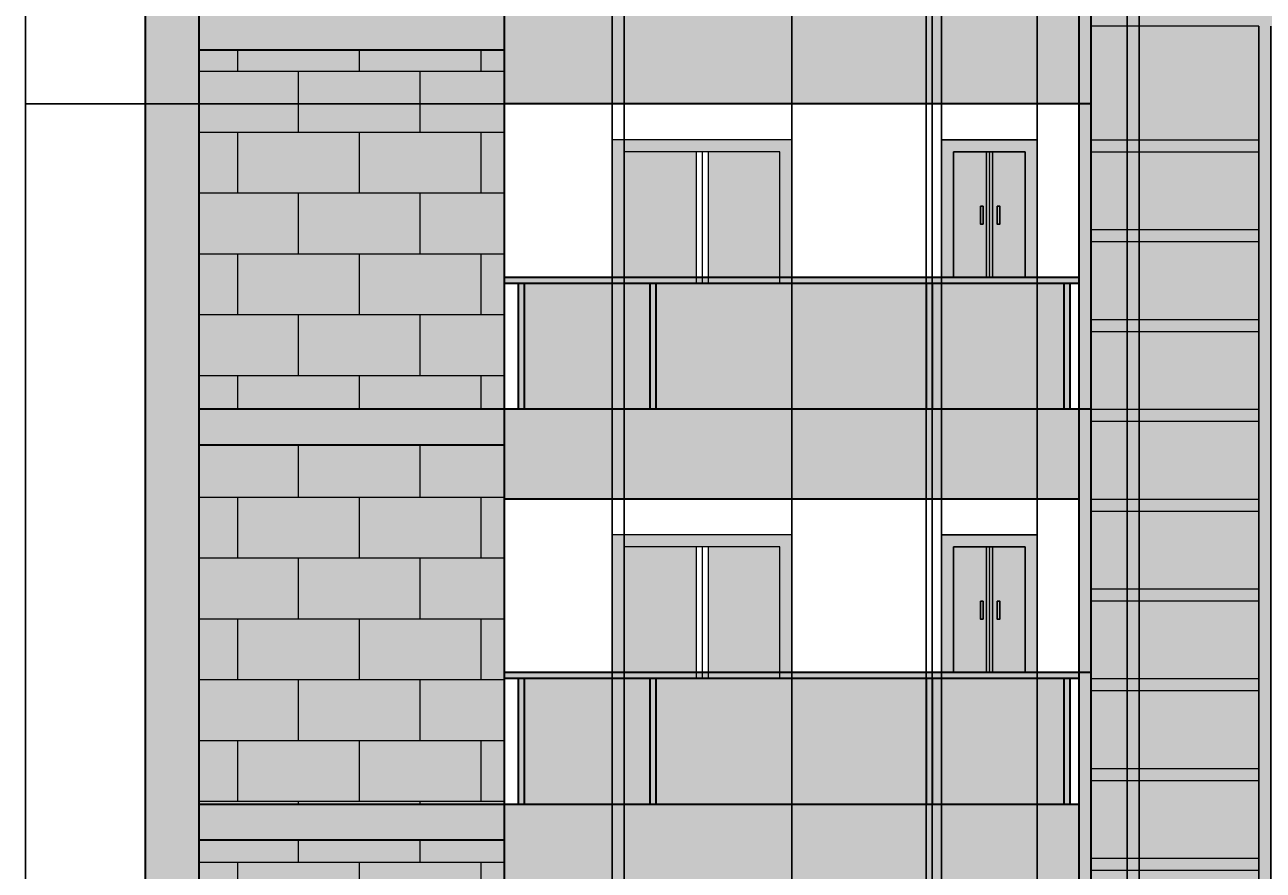
# Model space of a CAD drawing. Units: inches. Extents: x 2794 to 3619, y 522 to 1397.
# Tile 7 of 10: x 2794 to 3208, y 973 to 1255. Entities that reach past the tile are written whole.
import ezdxf

# ---------------------------------------------------------------- set-up
doc = ezdxf.new("R2010")
doc.units = ezdxf.units.IN
for name, color, linetype, lineweight in [('A-ANNO-DIMS', 2, 'Continuous', 18), ('A-DOOR', 3, 'Continuous', 25), ('A-ELEV', 7, 'Continuous', 35), ('A-ELEV-PATT', 8, 'Continuous', 13), ('A-GLAZ', 4, 'Continuous', 18)]:
    doc.layers.add(name, color=color, linetype=linetype, lineweight=lineweight)
doc.styles.get("Standard").update_dxf_attribs({"font": 'arial.ttf'})
doc.dimstyles.get("Standard").update_dxf_attribs({"dimtxt": 0.18, "dimasz": 0.18, "dimexe": 0.18, "dimexo": 0.0625, "dimgap": 0.09, "dimtad": 0, "dimtih": 1, "dimtoh": 1, "dimdec": 4, "dimzin": 0, "dimdsep": 46, "dimtxsty": 'Standard', "dimcen": 0.09, "dimadec": 0, "dimazin": 0, "dimtfac": 1, "dimtdec": 4, "dimtofl": 0, "dimtmove": 0, "dimatfit": 3, "dimfxl": 1, "dimtolj": 1, "dimtzin": 0, "dimarcsym": 0})

# ---------------------------------------------------------------- blocks, each defined once
blk = doc.blocks.new('WIN-1500')
at = {"transparency": 33554646}
h = blk.add_hatch(color=256, dxfattribs=at)
h.dxf.hatch_style = 1
h.paths.add_polyline_path([(60, 48), (0, 48), (0, 2), (4, 2), (4, 44), (56, 44), (56, 2), (60, 2)])
at = {"transparency": 33554687}
h = blk.add_hatch(color=256, dxfattribs=at)
h.dxf.hatch_style = 1
h.set_gradient(color1=(248, 246, 176), color2=(74, 13, 14), name='INVCYLINDER')
h.paths.add_polyline_path([(56, 44), (32, 44), (32, 2), (56, 2)])
h.paths.add_polyline_path([(28, 44), (4, 44), (4, 2), (28, 2)])
for p, q in [((0, 0), (0, 48)), ((60, 48), (0, 48)), ((60, 0), (60, 48)), ((56, 44), (4, 44)), ((4, 0), (4, 44)), ((28, 44), (28, 0)), ((30, 44), (30, 0)), ((32, 44), (32, 0)), ((56, 0), (56, 44))]:
    blk.add_line(p, q)
blk = doc.blocks.new('DOOR-BALCONY-DBL')
at = {"transparency": 33554628}
h = blk.add_hatch(color=256, dxfattribs=at)
h.dxf.hatch_style = 1
h.paths.add_polyline_path([(4, 42), (28, 42), (28, 0), (32, 0), (32, 46), (0, 46), (0, 0), (4, 0)])
at = {"transparency": 33554646}
h = blk.add_hatch(color=256, dxfattribs=at)
h.dxf.hatch_style = 1
h.set_gradient(color1=(255, 255, 255), color2=(147, 149, 152), name='INVCYLINDER')
h.paths.add_polyline_path([(15, 42), (4, 42), (4, 0), (15, 0)])
h = blk.add_hatch(color=256, dxfattribs=at)
h.dxf.hatch_style = 1
h.set_gradient(color1=(255, 255, 255), color2=(147, 149, 152), name='INVCYLINDER')
h.paths.add_polyline_path([(28, 42), (17, 42), (17, 0), (28, 0)])
for p, q in [((0, 0), (0, 46)), ((0, 46), (32, 46)), ((4, 46), (28, 46)), ((32, 0), (32, 46)), ((4, 0), (4, 42)), ((4, 42), (28, 42)), ((15, 0), (15, 42)), ((16, 0), (16, 42)), ((17, 0), (17, 42)), ((28, 0), (28, 42))]:
    blk.add_line(p, q)
for points in [[(12.99, 23.83), (13.93, 23.83), (13.93, 17.87), (12.99, 17.87)], [(18.59, 23.83), (19.53, 23.83), (19.53, 17.87), (18.59, 17.87)]]:
    blk.add_lwpolyline(points, close=True)
blk = doc.blocks.new('*D16')
at = {"layer": 'A-ANNO-DIMS', "color": 0, "lineweight": -2, "transparency": 16777216}
for p, q in [((3142.2, 1356.64), (2793.99, 1356.64)), ((2794.17, 1356.46), (2794.17, 959.82)), ((2794.17, 562.82), (2794.17, 959.45)), ((2834.2, 562.64), (2793.99, 562.64))]:
    blk.add_line(p, q, dxfattribs=at)
at = {"layer": 'A-ANNO-DIMS', "color": 0, "transparency": 16777216}
for points in [[(2794.14, 1356.46), (2794.2, 1356.46), (2794.17, 1356.64)], [(2794.14, 562.82), (2794.2, 562.82), (2794.17, 562.64)]]:
    blk.add_solid(points, dxfattribs=at)
at = {"layer": 'Defpoints', "color": 0, "transparency": 16777216}
for p in [(2794.17, 1356.64), (3142.27, 1356.64), (2834.27, 562.64)]:
    blk.add_point(p, dxfattribs=at)
at = {"layer": 'A-ANNO-DIMS', "color": 0, "transparency": 16777216, "insert": (2794.17, 959.64), "char_height": 0.18, "attachment_point": 5}
blk.add_mtext('\\A1;794', dxfattribs=at)
blk = doc.blocks.new('*D27')
at = {"layer": 'A-ANNO-DIMS', "color": 0, "lineweight": -2, "transparency": 16777216}
for p, q in [((2954.2, 1294.64), (2793.99, 1294.64)), ((2794.17, 1294.46), (2794.17, 1261.82)), ((2794.17, 1228.82), (2794.17, 1261.45)), ((2954.2, 1228.64), (2793.99, 1228.64))]:
    blk.add_line(p, q, dxfattribs=at)
at = {"layer": 'A-ANNO-DIMS', "color": 0, "transparency": 16777216}
for points in [[(2794.14, 1294.46), (2794.2, 1294.46), (2794.17, 1294.64)], [(2794.14, 1228.82), (2794.2, 1228.82), (2794.17, 1228.64)]]:
    blk.add_solid(points, dxfattribs=at)
at = {"layer": 'Defpoints', "color": 0, "transparency": 16777216}
for p in [(2794.17, 1294.64), (2954.27, 1294.64), (2954.27, 1228.64)]:
    blk.add_point(p, dxfattribs=at)
at = {"layer": 'A-ANNO-DIMS', "color": 0, "transparency": 16777216, "insert": (2794.17, 1261.64), "char_height": 0.18, "attachment_point": 5}
blk.add_mtext('\\A1;66', dxfattribs=at)
blk = doc.blocks.new('*D28')
at = {"layer": 'A-ANNO-DIMS', "color": 0, "lineweight": -2, "transparency": 16777216}
for p, q in [((2954.27, 832.7), (2954.27, 1396.92)), ((2954.45, 1396.74), (2972.05, 1396.74)), ((2990.09, 1396.74), (2972.48, 1396.74)), ((2990.27, 820.7), (2990.27, 1396.92))]:
    blk.add_line(p, q, dxfattribs=at)
at = {"layer": 'A-ANNO-DIMS', "color": 0, "transparency": 16777216}
for points in [[(2954.45, 1396.77), (2954.45, 1396.71), (2954.27, 1396.74)], [(2990.09, 1396.77), (2990.09, 1396.71), (2990.27, 1396.74)]]:
    blk.add_solid(points, dxfattribs=at)
at = {"layer": 'Defpoints', "color": 0, "transparency": 16777216}
for p in [(2990.27, 1396.74), (2954.27, 832.64), (2990.27, 820.64)]:
    blk.add_point(p, dxfattribs=at)
at = {"layer": 'A-ANNO-DIMS', "color": 0, "transparency": 16777216, "insert": (2972.27, 1396.74), "char_height": 0.18, "attachment_point": 5}
blk.add_mtext('\\A1;36', dxfattribs=at)
blk = doc.blocks.new('*D29')
at = {"layer": 'A-ANNO-DIMS', "color": 0, "lineweight": -2, "transparency": 16777216}
for p, q in [((2990.27, 820.7), (2990.27, 1396.92)), ((2990.45, 1396.74), (2992.11, 1396.74)), ((2994.09, 1396.74), (2992.42, 1396.74)), ((2994.27, 816.7), (2994.27, 1396.92))]:
    blk.add_line(p, q, dxfattribs=at)
at = {"layer": 'A-ANNO-DIMS', "color": 0, "transparency": 16777216}
for points in [[(2990.45, 1396.77), (2990.45, 1396.71), (2990.27, 1396.74)], [(2994.09, 1396.77), (2994.09, 1396.71), (2994.27, 1396.74)]]:
    blk.add_solid(points, dxfattribs=at)
at = {"layer": 'Defpoints', "color": 0, "transparency": 16777216}
for p in [(2994.27, 1396.74), (2990.27, 820.64), (2994.27, 816.64)]:
    blk.add_point(p, dxfattribs=at)
at = {"layer": 'A-ANNO-DIMS', "color": 0, "transparency": 16777216, "insert": (2992.27, 1396.74), "char_height": 0.18, "attachment_point": 5}
blk.add_mtext('\\A1;4', dxfattribs=at)
blk = doc.blocks.new('*D30')
at = {"layer": 'A-ANNO-DIMS', "color": 0, "lineweight": -2, "transparency": 16777216}
for p, q in [((3050.27, 820.7), (3050.27, 1396.92)), ((3050.45, 1396.74), (3075.05, 1396.74)), ((3100.09, 1396.74), (3075.48, 1396.74)), ((3100.27, 820.7), (3100.27, 1396.92))]:
    blk.add_line(p, q, dxfattribs=at)
at = {"layer": 'A-ANNO-DIMS', "color": 0, "transparency": 16777216}
for points in [[(3050.45, 1396.77), (3050.45, 1396.71), (3050.27, 1396.74)], [(3100.09, 1396.77), (3100.09, 1396.71), (3100.27, 1396.74)]]:
    blk.add_solid(points, dxfattribs=at)
at = {"layer": 'Defpoints', "color": 0, "transparency": 16777216}
for p in [(3100.27, 1396.74), (3050.27, 820.64), (3100.27, 820.64)]:
    blk.add_point(p, dxfattribs=at)
at = {"layer": 'A-ANNO-DIMS', "color": 0, "transparency": 16777216, "insert": (3075.27, 1396.74), "char_height": 0.18, "attachment_point": 5}
blk.add_mtext('\\A1;50', dxfattribs=at)
blk = doc.blocks.new('*D31')
at = {"layer": 'A-ANNO-DIMS', "color": 0, "lineweight": -2, "transparency": 16777216}
for p, q in [((3132.27, 820.7), (3132.27, 1396.92)), ((3132.45, 1396.74), (3139.06, 1396.74)), ((3146.09, 1396.74), (3139.48, 1396.74)), ((3146.27, 774.7), (3146.27, 1396.92))]:
    blk.add_line(p, q, dxfattribs=at)
at = {"layer": 'A-ANNO-DIMS', "color": 0, "transparency": 16777216}
for points in [[(3132.45, 1396.77), (3132.45, 1396.71), (3132.27, 1396.74)], [(3146.09, 1396.77), (3146.09, 1396.71), (3146.27, 1396.74)]]:
    blk.add_solid(points, dxfattribs=at)
at = {"layer": 'Defpoints', "color": 0, "transparency": 16777216}
for p in [(3146.27, 1396.74), (3132.27, 820.64), (3146.27, 774.64)]:
    blk.add_point(p, dxfattribs=at)
at = {"layer": 'A-ANNO-DIMS', "color": 0, "transparency": 16777216, "insert": (3139.27, 1396.74), "char_height": 0.18, "attachment_point": 5}
blk.add_mtext('\\A1;14', dxfattribs=at)
blk = doc.blocks.new('*D37')
at = {"layer": 'A-ANNO-DIMS', "color": 0, "lineweight": -2, "transparency": 16777216}
for p, q in [((3095.13, 772.7), (3095.13, 1396.92)), ((3095.31, 1396.74), (3095.98, 1396.74)), ((3096.95, 1396.74), (3096.28, 1396.74)), ((3097.13, 772.7), (3097.13, 1396.92))]:
    blk.add_line(p, q, dxfattribs=at)
at = {"layer": 'A-ANNO-DIMS', "color": 0, "transparency": 16777216}
for points in [[(3095.31, 1396.77), (3095.31, 1396.71), (3095.13, 1396.74)], [(3096.95, 1396.77), (3096.95, 1396.71), (3097.13, 1396.74)]]:
    blk.add_solid(points, dxfattribs=at)
at = {"layer": 'Defpoints', "color": 0, "transparency": 16777216}
for p in [(3097.13, 1396.74), (3095.13, 772.64), (3097.13, 772.64)]:
    blk.add_point(p, dxfattribs=at)
at = {"layer": 'A-ANNO-DIMS', "color": 0, "transparency": 16777216, "insert": (3096.13, 1396.74), "char_height": 0.18, "attachment_point": 5}
blk.add_mtext('\\A1;2', dxfattribs=at)
blk = doc.blocks.new('*D49')
at = {"layer": 'A-ANNO-DIMS', "color": 0, "lineweight": -2, "transparency": 16777216}
for p, q in [((3146.27, 1256.19), (3146.27, 522.36)), ((3150.27, 1254.57), (3150.27, 522.36)), ((3146.45, 522.54), (3148.11, 522.54)), ((3150.09, 522.54), (3148.42, 522.54))]:
    blk.add_line(p, q, dxfattribs=at)
at = {"layer": 'A-ANNO-DIMS', "color": 0, "transparency": 16777216}
for points in [[(3146.45, 522.57), (3146.45, 522.51), (3146.27, 522.54)], [(3150.09, 522.57), (3150.09, 522.51), (3150.27, 522.54)]]:
    blk.add_solid(points, dxfattribs=at)
at = {"layer": 'Defpoints', "color": 0, "transparency": 16777216}
for p in [(3146.27, 1256.25), (3150.27, 1254.64), (3150.27, 522.54)]:
    blk.add_point(p, dxfattribs=at)
at = {"layer": 'A-ANNO-DIMS', "color": 0, "transparency": 16777216, "insert": (3148.27, 522.54), "char_height": 0.18, "attachment_point": 5}
blk.add_mtext('\\A1;4', dxfattribs=at)
blk = doc.blocks.new('*D50')
at = {"layer": 'A-ANNO-DIMS', "color": 0, "lineweight": -2, "transparency": 16777216}
for p, q in [((3150.27, 1254.57), (3150.27, 522.36)), ((3206.27, 1254.57), (3206.27, 522.36)), ((3150.45, 522.54), (3178.05, 522.54)), ((3206.09, 522.54), (3178.48, 522.54))]:
    blk.add_line(p, q, dxfattribs=at)
at = {"layer": 'A-ANNO-DIMS', "color": 0, "transparency": 16777216}
for points in [[(3150.45, 522.57), (3150.45, 522.51), (3150.27, 522.54)], [(3206.09, 522.57), (3206.09, 522.51), (3206.27, 522.54)]]:
    blk.add_solid(points, dxfattribs=at)
at = {"layer": 'Defpoints', "color": 0, "transparency": 16777216}
for p in [(3150.27, 1254.64), (3206.27, 1254.64), (3206.27, 522.54)]:
    blk.add_point(p, dxfattribs=at)
at = {"layer": 'A-ANNO-DIMS', "color": 0, "transparency": 16777216, "insert": (3178.27, 522.54), "char_height": 0.18, "attachment_point": 5}
blk.add_mtext('\\A1;56', dxfattribs=at)
blk = doc.blocks.new('*D51')
at = {"layer": 'A-ANNO-DIMS', "color": 0, "lineweight": -2, "transparency": 16777216}
for p, q in [((3206.27, 1254.57), (3206.27, 522.36)), ((3210.27, 1254.57), (3210.27, 522.36)), ((3206.45, 522.54), (3208.11, 522.54)), ((3210.09, 522.54), (3208.42, 522.54))]:
    blk.add_line(p, q, dxfattribs=at)
at = {"layer": 'A-ANNO-DIMS', "color": 0, "transparency": 16777216}
for points in [[(3206.45, 522.57), (3206.45, 522.51), (3206.27, 522.54)], [(3210.09, 522.57), (3210.09, 522.51), (3210.27, 522.54)]]:
    blk.add_solid(points, dxfattribs=at)
at = {"layer": 'Defpoints', "color": 0, "transparency": 16777216}
for p in [(3206.27, 1254.64), (3210.27, 1254.64), (3210.27, 522.54)]:
    blk.add_point(p, dxfattribs=at)
at = {"layer": 'A-ANNO-DIMS', "color": 0, "transparency": 16777216, "insert": (3208.27, 522.54), "char_height": 0.18, "attachment_point": 5}
blk.add_mtext('\\A1;4', dxfattribs=at)
blk = doc.blocks.new('*D56')
at = {"layer": 'A-ANNO-DIMS', "color": 0, "lineweight": -2, "transparency": 16777216}
for p, q in [((3162.27, 664.7), (3162.27, 1396.92)), ((3162.45, 1396.74), (3206.05, 1396.74)), ((3250.09, 1396.74), (3206.49, 1396.74)), ((3250.27, 664.7), (3250.27, 1396.92))]:
    blk.add_line(p, q, dxfattribs=at)
at = {"layer": 'A-ANNO-DIMS', "color": 0, "transparency": 16777216}
for points in [[(3162.45, 1396.77), (3162.45, 1396.71), (3162.27, 1396.74)], [(3250.09, 1396.77), (3250.09, 1396.71), (3250.27, 1396.74)]]:
    blk.add_solid(points, dxfattribs=at)
at = {"layer": 'Defpoints', "color": 0, "transparency": 16777216}
for p in [(3250.27, 1396.74), (3162.27, 664.64), (3250.27, 664.64)]:
    blk.add_point(p, dxfattribs=at)
at = {"layer": 'A-ANNO-DIMS', "color": 0, "transparency": 16777216, "insert": (3206.27, 1396.74), "char_height": 0.18, "attachment_point": 5}
blk.add_mtext('\\A1;88', dxfattribs=at)
blk = doc.blocks.new('*D57')
at = {"layer": 'A-ANNO-DIMS', "color": 0, "lineweight": -2, "transparency": 16777216}
for p, q in [((3162.27, 664.7), (3162.27, 1396.92)), ((3162.45, 1396.74), (3164.11, 1396.74)), ((3166.09, 1396.74), (3164.42, 1396.74)), ((3166.27, 660.7), (3166.27, 1396.92))]:
    blk.add_line(p, q, dxfattribs=at)
at = {"layer": 'A-ANNO-DIMS', "color": 0, "transparency": 16777216}
for points in [[(3162.45, 1396.77), (3162.45, 1396.71), (3162.27, 1396.74)], [(3166.09, 1396.77), (3166.09, 1396.71), (3166.27, 1396.74)]]:
    blk.add_solid(points, dxfattribs=at)
at = {"layer": 'Defpoints', "color": 0, "transparency": 16777216}
for p in [(3166.27, 1396.74), (3162.27, 664.64), (3166.27, 660.64)]:
    blk.add_point(p, dxfattribs=at)
at = {"layer": 'A-ANNO-DIMS', "color": 0, "transparency": 16777216, "insert": (3164.27, 1396.74), "char_height": 0.18, "attachment_point": 5}
blk.add_mtext('\\A1;4', dxfattribs=at)
blk = doc.blocks.new('*D58')
at = {"layer": 'A-ANNO-DIMS', "color": 0, "lineweight": -2, "transparency": 16777216}
for p, q in [((3150.27, 580.7), (3150.27, 1396.92)), ((3150.45, 1396.74), (3156.06, 1396.74)), ((3162.09, 1396.74), (3156.48, 1396.74)), ((3162.27, 664.7), (3162.27, 1396.92))]:
    blk.add_line(p, q, dxfattribs=at)
at = {"layer": 'A-ANNO-DIMS', "color": 0, "transparency": 16777216}
for points in [[(3150.45, 1396.77), (3150.45, 1396.71), (3150.27, 1396.74)], [(3162.09, 1396.77), (3162.09, 1396.71), (3162.27, 1396.74)]]:
    blk.add_solid(points, dxfattribs=at)
at = {"layer": 'Defpoints', "color": 0, "transparency": 16777216}
for p in [(3162.27, 1396.74), (3162.27, 664.64), (3150.27, 580.64)]:
    blk.add_point(p, dxfattribs=at)
at = {"layer": 'A-ANNO-DIMS', "color": 0, "transparency": 16777216, "insert": (3156.27, 1396.74), "char_height": 0.18, "attachment_point": 5}
blk.add_mtext('\\A1;12', dxfattribs=at)

msp = doc.modelspace()

# ---------------------------------------------------------------- hatches: boundary and pattern name
at = {"layer": 'A-ELEV-PATT', "transparency": 33554687}
h = msp.add_hatch(color=256, dxfattribs=at)
h.dxf.hatch_style = 1
h.paths.add_polyline_path([(3262.2659, 1350.6351), (3150.2659, 1350.6351), (3150.2659, 1279.0155, -0.68639605), (3262.2659, 1279.0155)])
h.paths.add_polyline_path([(3210.2659, 1314.1121), (3210.2659, 1258.6351), (3262.2659, 1258.6351, 0.39146256)])
h.paths.add_polyline_path([(3206.2659, 1314.2551, 0.41222069), (3150.2659, 1258.6351), (3206.2659, 1258.6351)])
h.paths.add_polyline_path([(3262.2659, 1254.6351), (3210.2659, 1254.6351), (3210.2659, 1216.6351), (3262.2659, 1216.6351)])
h.paths.add_polyline_path([(3206.2659, 1254.6351), (3150.2659, 1254.6351), (3150.2659, 1216.6351), (3206.2659, 1216.6351)])
h.paths.add_polyline_path([(3262.2659, 1212.6351), (3210.2659, 1212.6351), (3210.2659, 1186.6351), (3262.2659, 1186.6351)])
h.paths.add_polyline_path([(3206.2659, 1212.6351), (3150.2659, 1212.6351), (3150.2659, 1186.6351), (3206.2659, 1186.6351)])
h.paths.add_polyline_path([(3206.2659, 1182.6351), (3150.2659, 1182.6351), (3150.2659, 1156.6351), (3206.2659, 1156.6351)])
h.paths.add_polyline_path([(3262.2659, 1182.6351), (3210.2659, 1182.6351), (3210.2659, 1156.6351), (3262.2659, 1156.6351)])
h.paths.add_polyline_path([(3262.2659, 1152.6351), (3210.2659, 1152.6351), (3210.2659, 1126.6351), (3262.2659, 1126.6351)])
h.paths.add_polyline_path([(3206.2659, 1152.6351), (3150.2659, 1152.6351), (3150.2659, 1126.6351), (3206.2659, 1126.6351)])
h.paths.add_polyline_path([(3262.2659, 1122.6351), (3210.2659, 1122.6351), (3210.2659, 1096.6351), (3262.2659, 1096.6351)])
h.paths.add_polyline_path([(3206.2659, 1122.6351), (3150.2659, 1122.6351), (3150.2659, 1096.6351), (3206.2659, 1096.6351)])
h.paths.add_polyline_path([(3206.2659, 1092.6351), (3150.2659, 1092.6351), (3150.2659, 1066.6351), (3206.2659, 1066.6351)])
h.paths.add_polyline_path([(3262.2659, 1092.6351), (3210.2659, 1092.6351), (3210.2659, 1066.6351), (3262.2659, 1066.6351)])
h.paths.add_polyline_path([(3262.2659, 1062.6351), (3210.2659, 1062.6351), (3210.2659, 1036.6351), (3262.2659, 1036.6351)])
h.paths.add_polyline_path([(3206.2659, 1062.6351), (3150.2659, 1062.6351), (3150.2659, 1036.6351), (3206.2659, 1036.6351)])
h.paths.add_polyline_path([(3206.2659, 1032.6351), (3150.2659, 1032.6351), (3150.2659, 1006.6351), (3206.2659, 1006.6351)])
h.paths.add_polyline_path([(3262.2659, 1032.6351), (3210.2659, 1032.6351), (3210.2659, 1006.6351), (3262.2659, 1006.6351)])
h.paths.add_polyline_path([(3262.2659, 1002.6351), (3210.2659, 1002.6351), (3210.2659, 976.6351), (3262.2659, 976.6351)])
h.paths.add_polyline_path([(3206.2659, 1002.6351), (3150.2659, 1002.6351), (3150.2659, 976.6351), (3206.2659, 976.6351)])
h.paths.add_polyline_path([(3206.2659, 972.6351), (3150.2659, 972.6351), (3150.2659, 946.6351), (3206.2659, 946.6351)])
h.paths.add_polyline_path([(3206.2659, 942.6351), (3150.2659, 942.6351), (3150.2659, 916.6351), (3206.2659, 916.6351)])
h.paths.add_polyline_path([(3262.2659, 942.6351), (3210.2659, 942.6351), (3210.2659, 916.6351), (3262.2659, 916.6351)])
h.paths.add_polyline_path([(3262.2659, 972.6351), (3210.2659, 972.6351), (3210.2659, 946.6351), (3262.2659, 946.6351)])
h.paths.add_polyline_path([(3262.2659, 912.6351), (3210.2659, 912.6351), (3210.2659, 886.6351), (3262.2659, 886.6351)])
h.paths.add_polyline_path([(3206.2659, 912.6351), (3150.2659, 912.6351), (3150.2659, 886.6351), (3206.2659, 886.6351)])
h.paths.add_polyline_path([(3206.2659, 882.6351), (3150.2659, 882.6351), (3150.2659, 856.6351), (3206.2659, 856.6351)])
h.paths.add_polyline_path([(3262.2659, 882.6351), (3210.2659, 882.6351), (3210.2659, 856.6351), (3262.2659, 856.6351)])
h.paths.add_polyline_path([(3262.2659, 852.6351), (3210.2659, 852.6351), (3210.2659, 826.6351), (3262.2659, 826.6351)])
h.paths.add_polyline_path([(3206.2659, 852.6351), (3150.2659, 852.6351), (3150.2659, 826.6351), (3206.2659, 826.6351)])
h.paths.add_polyline_path([(3206.2659, 822.6351), (3150.2659, 822.6351), (3150.2659, 796.6351), (3206.2659, 796.6351)])
h.paths.add_polyline_path([(3262.2659, 822.6351), (3210.2659, 822.6351), (3210.2659, 796.6351), (3262.2659, 796.6351)])
h.paths.add_polyline_path([(3262.2659, 792.6351), (3210.2659, 792.6351), (3210.2659, 766.6351), (3262.2659, 766.6351)])
h.paths.add_polyline_path([(3206.2659, 792.6351), (3150.2659, 792.6351), (3150.2659, 766.6351), (3206.2659, 766.6351)])
h.paths.add_polyline_path([(3206.2659, 762.6351), (3150.2659, 762.6351), (3150.2659, 736.6351), (3206.2659, 736.6351)])
h.paths.add_polyline_path([(3206.2659, 732.6351), (3150.2659, 732.6351), (3150.2659, 706.6351), (3206.2659, 706.6351)])
h.paths.add_polyline_path([(3262.2659, 732.6351), (3210.2659, 732.6351), (3210.2659, 706.6351), (3262.2659, 706.6351)])
h.paths.add_polyline_path([(3262.2659, 762.6351), (3210.2659, 762.6351), (3210.2659, 736.6351), (3262.2659, 736.6351)])
h = msp.add_hatch(color=256, dxfattribs=at)
h.dxf.hatch_style = 1
h.paths.add_polyline_path([(3150.2659, 1257.8725, -0.00340445), (3150.2659, 1258.6351), (3146.2659, 1258.6351), (3146.2659, 1228.6351), (3150.2659, 1228.6351)])
h.paths.add_polyline_path([(3262.2659, 1258.6351), (3210.2659, 1258.6351), (3210.2659, 1314.1121, 0.01787385), (3206.2659, 1314.2551), (3206.2659, 1258.6351), (3150.2659, 1258.6351), (3150.2659, 1254.6351), (3206.2659, 1254.6351), (3206.2659, 1216.6351), (3150.2659, 1216.6351), (3150.2659, 1212.6351), (3206.2659, 1212.6351), (3206.2659, 1186.6351), (3150.2659, 1186.6351), (3150.2659, 1182.6351), (3206.2659, 1182.6351), (3206.2659, 1156.6351), (3150.2659, 1156.6351), (3150.2659, 1152.6351), (3206.2659, 1152.6351), (3206.2659, 1126.6351), (3150.2659, 1126.6351), (3150.2659, 1122.6351), (3206.2659, 1122.6351), (3206.2659, 1096.6351), (3150.2659, 1096.6351), (3150.2659, 1092.6351), (3206.2659, 1092.6351), (3206.2659, 1066.6351), (3150.2659, 1066.6351), (3150.2659, 1062.6351), (3206.2659, 1062.6351), (3206.2659, 1036.6351), (3150.2659, 1036.6351), (3150.2659, 1032.6351), (3206.2659, 1032.6351), (3206.2659, 1006.6351), (3150.2659, 1006.6351), (3150.2659, 1002.6351), (3206.2659, 1002.6351), (3206.2659, 976.6351), (3150.2659, 976.6351), (3150.2659, 972.6351), (3206.2659, 972.6351), (3206.2659, 946.6351), (3150.2659, 946.6351), (3150.2659, 942.6351), (3206.2659, 942.6351), (3206.2659, 916.6351), (3150.2659, 916.6351), (3150.2659, 912.6351), (3206.2659, 912.6351), (3206.2659, 886.6351), (3150.2659, 886.6351), (3150.2659, 882.6351), (3206.2659, 882.6351), (3206.2659, 856.6351), (3150.2659, 856.6351), (3150.2659, 852.6351), (3206.2659, 852.6351), (3206.2659, 826.6351), (3150.2659, 826.6351), (3150.2659, 822.6351), (3206.2659, 822.6351), (3206.2659, 796.6351), (3150.2659, 796.6351), (3150.2659, 792.6351), (3206.2659, 792.6351), (3206.2659, 766.6351), (3150.2659, 766.6351), (3150.2659, 762.6351), (3206.2659, 762.6351), (3206.2659, 736.6351), (3150.2659, 736.6351), (3150.2659, 732.6351), (3206.2659, 732.6351), (3206.2659, 706.6351), (3150.2659, 706.6351), (3150.2659, 702.6351), (3262.2659, 702.6351), (3262.2659, 706.6351), (3210.2659, 706.6351), (3210.2659, 732.6351), (3262.2659, 732.6351), (3262.2659, 736.6351), (3210.2659, 736.6351), (3210.2659, 762.6351), (3262.2659, 762.6351), (3262.2659, 766.6351), (3210.2659, 766.6351), (3210.2659, 792.6351), (3262.2659, 792.6351), (3262.2659, 796.6351), (3210.2659, 796.6351), (3210.2659, 822.6351), (3262.2659, 822.6351), (3262.2659, 826.6351), (3210.2659, 826.6351), (3210.2659, 852.6351), (3262.2659, 852.6351), (3262.2659, 856.6351), (3210.2659, 856.6351), (3210.2659, 882.6351), (3262.2659, 882.6351), (3262.2659, 886.6351), (3210.2659, 886.6351), (3210.2659, 912.6351), (3262.2659, 912.6351), (3262.2659, 916.6351), (3210.2659, 916.6351), (3210.2659, 942.6351), (3262.2659, 942.6351), (3262.2659, 946.6351), (3210.2659, 946.6351), (3210.2659, 972.6351), (3262.2659, 972.6351), (3262.2659, 976.6351), (3210.2659, 976.6351), (3210.2659, 1002.6351), (3262.2659, 1002.6351), (3262.2659, 1006.6351), (3210.2659, 1006.6351), (3210.2659, 1032.6351), (3262.2659, 1032.6351), (3262.2659, 1036.6351), (3210.2659, 1036.6351), (3210.2659, 1062.6351), (3262.2659, 1062.6351), (3262.2659, 1066.6351), (3210.2659, 1066.6351), (3210.2659, 1092.6351), (3262.2659, 1092.6351), (3262.2659, 1096.6351), (3210.2659, 1096.6351), (3210.2659, 1122.6351), (3262.2659, 1122.6351), (3262.2659, 1126.6351), (3210.2659, 1126.6351), (3210.2659, 1152.6351), (3262.2659, 1152.6351), (3262.2659, 1156.6351), (3210.2659, 1156.6351), (3210.2659, 1182.6351), (3262.2659, 1182.6351), (3262.2659, 1186.6351), (3210.2659, 1186.6351), (3210.2659, 1212.6351), (3262.2659, 1212.6351), (3262.2659, 1216.6351), (3210.2659, 1216.6351), (3210.2659, 1254.6351), (3262.2659, 1254.6351)])
h = msp.add_hatch(color=256, dxfattribs=at)
h.dxf.hatch_style = 1
h.paths.add_polyline_path([(3578.2659, 1294.6351), (3560.2659, 1294.6351), (3560.2659, 642.6351), (3578.2659, 642.6351)])
h.paths.add_polyline_path([(2852.2659, 1294.6351), (2834.2659, 1294.6351), (2834.2659, 642.6351), (2852.2659, 642.6351)])
h = msp.add_hatch(color=256, dxfattribs=at)
h.dxf.hatch_style = 1
h.paths.add_polyline_path([(2852.2659, 1294.6351), (2834.2659, 1294.6351), (2834.2659, 562.6351), (2852.2659, 562.6351)])
h.paths.add_polyline_path([(3578.2659, 1294.6351), (3560.2659, 1294.6351), (3560.2659, 562.6351), (3578.2659, 562.6351)])
h = msp.add_hatch(color=256, dxfattribs=at)
h.dxf.hatch_style = 1
h.paths.add_polyline_path([(2852.2659, 1246.6351), (2954.2659, 1246.6351), (2954.2659, 1258.6351), (2900.2659, 1258.6351), (2900.2659, 1294.6351), (2852.2659, 1294.6351)])
h.paths.add_polyline_path([(3512.2659, 1294.6351), (3512.2659, 1258.6351), (3458.2659, 1258.6351), (3458.2659, 1246.6351), (3560.2659, 1246.6351), (3560.2659, 1294.6351)])
h.paths.add_polyline_path([(2954.2659, 1114.6351), (2954.2659, 1126.6351), (2852.2659, 1126.6351), (2852.2659, 1114.6351)])
h.paths.add_polyline_path([(3560.2659, 1114.6351), (3560.2659, 1126.6351), (3458.2659, 1126.6351), (3458.2659, 1114.6351)])
h.paths.add_polyline_path([(3560.2659, 982.6351), (3560.2659, 994.6351), (3458.2659, 994.6351), (3458.2659, 982.6351)])
h.paths.add_polyline_path([(2954.2659, 982.6351), (2954.2659, 994.6351), (2852.2659, 994.6351), (2852.2659, 982.6351)])
h.paths.add_polyline_path([(2852.2659, 862.6351), (2852.2659, 850.6351), (2954.2659, 850.6351), (2954.2659, 862.6351)])
h.paths.add_polyline_path([(2852.2659, 730.6351), (2852.2659, 718.6351), (2954.2659, 718.6351), (2954.2659, 730.6351)])
h.paths.add_polyline_path([(3560.2659, 718.6351), (3560.2659, 730.6351), (3458.2659, 730.6351), (3458.2659, 718.6351)])
h.paths.add_polyline_path([(3560.2659, 850.6351), (3560.2659, 862.6351), (3458.2659, 862.6351), (3458.2659, 850.6351)])
h = msp.add_hatch(color=256, dxfattribs=at)
h.dxf.hatch_style = 1
h.paths.add_polyline_path([(3146.2659, 1096.6351), (3146.2659, 1126.6351), (2954.2659, 1126.6351), (2954.2659, 1096.6351)])
h.paths.add_polyline_path([(3458.2659, 1096.6351), (3458.2659, 1126.6351), (3266.2659, 1126.6351), (3266.2659, 1096.6351)])
h.paths.add_polyline_path([(3458.2659, 964.6351), (3458.2659, 994.6351), (3266.2659, 994.6351), (3266.2659, 964.6351)])
h.paths.add_polyline_path([(3146.2659, 964.6351), (3146.2659, 994.6351), (2954.2659, 994.6351), (2954.2659, 964.6351)])
h.paths.add_polyline_path([(3458.2659, 832.6351), (3458.2659, 862.6351), (3266.2659, 862.6351), (3266.2659, 832.6351)])
h.paths.add_polyline_path([(3146.2659, 832.6351), (3146.2659, 862.6351), (2954.2659, 862.6351), (2954.2659, 832.6351)])
h.paths.add_polyline_path([(3458.2659, 700.6351), (3458.2659, 730.6351), (3266.2659, 730.6351), (3266.2659, 700.6351)])
h.paths.add_polyline_path([(3146.2659, 700.6351), (3146.2659, 730.6351), (2954.2659, 730.6351), (2954.2659, 700.6351)])
h.paths.add_polyline_path([(3266.2659, 1294.6351), (3266.2659, 1258.6351), (3266.2659, 1228.6351), (3458.2659, 1228.6351), (3458.2659, 1294.6351)])
h.paths.add_polyline_path([(3146.2659, 1228.6351), (3146.2659, 1256.2485, -0.00994307), (3146.2659, 1258.6351), (3146.2659, 1294.6351), (2954.2659, 1294.6351), (2954.2659, 1228.6351)])
at = {"layer": 'A-ELEV-PATT'}
h = msp.add_hatch(dxfattribs=at)
h.set_pattern_fill('AR-B816', color=256, scale=0.1)
h.paths.add_polyline_path([(2954.2659, 1114.6351), (2852.2659, 1114.6351), (2852.2659, 994.6351), (2954.2659, 994.6351)])
h.paths.add_polyline_path([(2954.2659, 1246.6351), (2852.2659, 1246.6351), (2852.2659, 1126.6351), (2954.2659, 1126.6351)])
h.paths.add_polyline_path([(2954.2659, 982.6351), (2852.2659, 982.6351), (2852.2659, 862.6351), (2954.2659, 862.6351)])
h.paths.add_polyline_path([(2954.2659, 850.6351), (2852.2659, 850.6351), (2852.2659, 730.6351), (2954.2659, 730.6351)])
h.paths.add_polyline_path([(3560.2659, 850.6351), (3458.2659, 850.6351), (3458.2659, 730.6351), (3560.2659, 730.6351)])
h.paths.add_polyline_path([(3560.2659, 982.6351), (3458.2659, 982.6351), (3458.2659, 862.6351), (3560.2659, 862.6351)])
h.paths.add_polyline_path([(3560.2659, 1114.6351), (3458.2659, 1114.6351), (3458.2659, 994.6351), (3560.2659, 994.6351)])
h.paths.add_polyline_path([(3560.2659, 1246.6351), (3458.2659, 1246.6351), (3458.2659, 1126.6351), (3560.2659, 1126.6351)])
h.paths.add_polyline_path([(2852.2659, 642.6351), (2954.2659, 642.6351), (2954.2659, 718.6351), (2852.2659, 718.6351)])
h.paths.add_polyline_path([(3458.2659, 640.6351), (3560.2659, 640.6351), (3560.2659, 718.6351), (3458.2659, 718.6351)])
at = {"layer": 'A-ELEV-PATT', "transparency": 33554630}
h = msp.add_hatch(color=256, dxfattribs=at)
h.dxf.hatch_style = 1
h.paths.add_polyline_path([(2954.2659, 1246.6351), (2852.2659, 1246.6351), (2852.2659, 1126.6351), (2954.2659, 1126.6351)])
h = msp.add_hatch(color=256, dxfattribs=at)
h.dxf.hatch_style = 1
h.paths.add_polyline_path([(2954.2659, 1114.6351), (2852.2659, 1114.6351), (2852.2659, 994.6351), (2954.2659, 994.6351)])
h.paths.add_polyline_path([(2954.2659, 982.6351), (2852.2659, 982.6351), (2852.2659, 862.6351), (2954.2659, 862.6351)])
h.paths.add_polyline_path([(2954.2659, 850.6351), (2852.2659, 850.6351), (2852.2659, 730.6351), (2954.2659, 730.6351)])
h.paths.add_polyline_path([(3560.2659, 850.6351), (3458.2659, 850.6351), (3458.2659, 730.6351), (3560.2659, 730.6351)])
h.paths.add_polyline_path([(3560.2659, 982.6351), (3458.2659, 982.6351), (3458.2659, 862.6351), (3560.2659, 862.6351)])
h.paths.add_polyline_path([(3560.2659, 1114.6351), (3458.2659, 1114.6351), (3458.2659, 994.6351), (3560.2659, 994.6351)])
h.paths.add_polyline_path([(3560.2659, 1246.6351), (3458.2659, 1246.6351), (3458.2659, 1126.6351), (3560.2659, 1126.6351)])
h.paths.add_polyline_path([(2852.2659, 642.6351), (2954.2659, 642.6351), (2954.2659, 718.6351), (2852.2659, 718.6351)])
h.paths.add_polyline_path([(3458.2659, 642.6351), (3560.2659, 642.6351), (3560.2659, 718.6351), (3458.2659, 718.6351)])
at = {"layer": 'A-ELEV-PATT', "transparency": 33554687}
h = msp.add_hatch(color=256, dxfattribs=at)
h.dxf.hatch_style = 1
h.paths.add_polyline_path([(3150.2659, 1228.6351), (3146.2659, 1228.6351), (3146.2659, 1126.6351), (3150.2659, 1126.6351)])
h.paths.add_polyline_path([(3150.2659, 1126.6351), (3146.2659, 1126.6351), (3146.2659, 1038.6351), (3150.2659, 1038.6351)])
h.paths.add_polyline_path([(3150.2659, 1038.6351), (3146.2659, 1038.6351), (3146.2659, 964.6351), (3150.2659, 964.6351)])
h.paths.add_polyline_path([(3150.2659, 964.6351), (3146.2659, 964.6351), (3146.2659, 906.6351), (3150.2659, 906.6351)])
h.paths.add_polyline_path([(3150.2659, 906.6351), (3146.2659, 906.6351), (3146.2659, 832.6351), (3150.2659, 832.6351)])
h.paths.add_polyline_path([(3150.2659, 832.6351), (3146.2659, 832.6351), (3146.2659, 730.6351), (3150.2659, 730.6351)])
h = msp.add_hatch(color=256, dxfattribs=at)
h.dxf.hatch_style = 1
h.paths.add_polyline_path([(3097.1329, 904.6351), (3095.1329, 904.6351), (3095.1329, 862.6351), (3097.1329, 862.6351)])
h.paths.add_polyline_path([(3143.112, 904.6351), (3141.112, 904.6351), (3141.112, 862.6351), (3143.112, 862.6351)])
h.paths.add_polyline_path([(3146.2659, 906.6351), (2954.2659, 906.6351), (2954.2659, 904.6351), (3146.2659, 904.6351)])
h.paths.add_polyline_path([(3004.8268, 904.6351), (3002.8268, 904.6351), (3002.8268, 862.6351), (3004.8268, 862.6351)])
h.paths.add_polyline_path([(2960.8268, 904.6351), (2958.8268, 904.6351), (2958.8268, 862.6351), (2960.8268, 862.6351)])
h.paths.add_polyline_path([(3146.2659, 1038.6351), (2954.2659, 1038.6351), (2954.2659, 1036.6351), (3146.2659, 1036.6351)])
h.paths.add_polyline_path([(2960.8268, 1036.6351), (2958.8268, 1036.6351), (2958.8268, 994.6351), (2960.8268, 994.6351)])
h.paths.add_polyline_path([(3004.8268, 1036.6351), (3002.8268, 1036.6351), (3002.8268, 994.6351), (3004.8268, 994.6351)])
h.paths.add_polyline_path([(3143.112, 1036.6351), (3141.112, 1036.6351), (3141.112, 994.6351), (3143.112, 994.6351)])
h.paths.add_polyline_path([(3097.1329, 1036.6351), (3095.1329, 1036.6351), (3095.1329, 994.6351), (3097.1329, 994.6351)])
h.paths.add_polyline_path([(3146.2659, 1170.6351), (2954.2659, 1170.6351), (2954.2659, 1168.6351), (3146.2659, 1168.6351)])
h.paths.add_polyline_path([(3004.8268, 1168.6351), (3002.8268, 1168.6351), (3002.8268, 1126.6351), (3004.8268, 1126.6351)])
h.paths.add_polyline_path([(2960.8268, 1168.6351), (2958.8268, 1168.6351), (2958.8268, 1126.6351), (2960.8268, 1126.6351)])
h.paths.add_polyline_path([(3143.112, 1168.6351), (3141.112, 1168.6351), (3141.112, 1126.6351), (3143.112, 1126.6351)])
h.paths.add_polyline_path([(3097.1329, 1168.6351), (3095.1329, 1168.6351), (3095.1329, 1126.6351), (3097.1329, 1126.6351)])
h.paths.add_polyline_path([(3458.2659, 1170.6351), (3266.2659, 1170.6351), (3266.2659, 1168.6351), (3458.2659, 1168.6351)])
h.paths.add_polyline_path([(3272.407, 1168.6351), (3270.407, 1168.6351), (3270.407, 1126.6351), (3272.407, 1126.6351)])
h.paths.add_polyline_path([(3316.407, 1168.6351), (3314.407, 1168.6351), (3314.407, 1126.6351), (3316.407, 1126.6351)])
h.paths.add_polyline_path([(3408.7131, 1168.6351), (3406.7131, 1168.6351), (3406.7131, 1126.6351), (3408.7131, 1126.6351)])
at = {"layer": 'A-GLAZ', "transparency": 33554556}
h = msp.add_hatch(color=256, dxfattribs=at)
h.dxf.hatch_style = 1
h.set_gradient(color1=(255, 255, 255), color2=(0, 255, 255), name='INVCYLINDER')
h.paths.add_polyline_path([(3002.8268, 1168.6351), (2960.8268, 1168.6351), (2960.8268, 1126.6351), (3002.8268, 1126.6351)])
h = msp.add_hatch(color=256, dxfattribs=at)
h.dxf.hatch_style = 1
h.set_gradient(color1=(255, 255, 255), color2=(0, 255, 255), name='INVCYLINDER')
h.paths.add_polyline_path([(3095.1329, 1168.6351), (3004.8268, 1168.6351), (3004.8268, 1126.6351), (3095.1329, 1126.6351)])
h = msp.add_hatch(color=256, dxfattribs=at)
h.dxf.hatch_style = 1
h.set_gradient(color1=(255, 255, 255), color2=(0, 255, 255), name='INVCYLINDER')
h.paths.add_polyline_path([(3141.112, 1168.6351), (3097.1329, 1168.6351), (3097.1329, 1126.6351), (3141.112, 1126.6351)])
h = msp.add_hatch(color=256, dxfattribs=at)
h.dxf.hatch_style = 1
h.set_gradient(color1=(255, 255, 255), color2=(0, 255, 255), name='INVCYLINDER')
h.paths.add_polyline_path([(3002.8268, 1036.6351), (2960.8268, 1036.6351), (2960.8268, 994.6351), (3002.8268, 994.6351)])
h = msp.add_hatch(color=256, dxfattribs=at)
h.dxf.hatch_style = 1
h.set_gradient(color1=(255, 255, 255), color2=(0, 255, 255), name='INVCYLINDER')
h.paths.add_polyline_path([(3095.1329, 1036.6351), (3004.8268, 1036.6351), (3004.8268, 994.6351), (3095.1329, 994.6351)])
h = msp.add_hatch(color=256, dxfattribs=at)
h.dxf.hatch_style = 1
h.set_gradient(color1=(255, 255, 255), color2=(0, 255, 255), name='INVCYLINDER')
h.paths.add_polyline_path([(3141.112, 1036.6351), (3097.1329, 1036.6351), (3097.1329, 994.6351), (3141.112, 994.6351)])

# ---------------------------------------------------------------- linework, layer by layer
at = {"layer": 'A-ELEV'}
for p, q in [((2834.2659, 562.6351), (2834.2659, 1297.6351)), ((2852.2659, 562.6351), (2852.2659, 1294.6351)), ((2954.2659, 598.6351), (2954.2659, 1294.6351)), ((3146.2659, 598.6351), (3146.2659, 1258.6351)), ((3150.2659, 598.6351), (3150.2659, 1258.6351)), ((2954.2659, 1246.6351), (2852.2659, 1246.6351)), ((3150.2659, 1228.6351), (2954.2659, 1228.6351)), ((3146.2659, 1170.6351), (2954.2659, 1170.6351)), ((3146.2659, 1168.6351), (2954.2659, 1168.6351)), ((2958.8268, 1168.6351), (2958.8268, 1126.6351)), ((2960.8268, 1168.6351), (2960.8268, 1126.6351)), ((3002.8268, 1168.6351), (3002.8268, 1126.6351)), ((3004.8268, 1168.6351), (3004.8268, 1126.6351)), ((3095.1329, 1168.6351), (3095.1329, 1126.6351)), ((3097.1329, 1168.6351), (3097.1329, 1126.6351)), ((3141.112, 1168.6351), (3141.112, 1126.6351)), ((3143.112, 1168.6351), (3143.112, 1126.6351)), ((3150.2659, 1126.6351), (2852.2659, 1126.6351)), ((2954.2659, 1114.6351), (2852.2659, 1114.6351)), ((3146.2659, 1096.6351), (2954.2659, 1096.6351)), ((3150.2659, 1038.6351), (2954.2659, 1038.6351)), ((3146.2659, 1036.6351), (2954.2659, 1036.6351)), ((2958.8268, 1036.6351), (2958.8268, 994.6351)), ((2960.8268, 1036.6351), (2960.8268, 994.6351)), ((3002.8268, 1036.6351), (3002.8268, 994.6351)), ((3004.8268, 1036.6351), (3004.8268, 994.6351)), ((3095.1329, 1036.6351), (3095.1329, 994.6351)), ((3097.1329, 1036.6351), (3097.1329, 994.6351)), ((3141.112, 1036.6351), (3141.112, 994.6351)), ((3143.112, 1036.6351), (3143.112, 994.6351)), ((3146.2659, 994.6351), (2852.2659, 994.6351)), ((2954.2659, 982.6351), (2852.2659, 982.6351))]:
    msp.add_line(p, q, dxfattribs=at)
at = {"layer": 'A-GLAZ'}
for p, q in [((3206.2659, 1254.6351), (3150.2659, 1254.6351)), ((3206.2659, 1254.6351), (3206.2659, 1216.6351)), ((3150.2659, 1216.6351), (3206.2659, 1216.6351)), ((3150.2659, 1212.6351), (3206.2659, 1212.6351)), ((3206.2659, 1212.6351), (3206.2659, 1186.6351)), ((3150.2659, 1186.6351), (3206.2659, 1186.6351)), ((3150.2659, 1182.6351), (3206.2659, 1182.6351)), ((3206.2659, 1182.6351), (3206.2659, 1156.6351)), ((3150.2659, 1156.6351), (3206.2659, 1156.6351)), ((3150.2659, 1152.6351), (3206.2659, 1152.6351)), ((3206.2659, 1152.6351), (3206.2659, 1126.6351)), ((3150.2659, 1126.6351), (3206.2659, 1126.6351)), ((3150.2659, 1122.6351), (3206.2659, 1122.6351)), ((3206.2659, 1122.6351), (3206.2659, 1096.6351)), ((3150.2659, 1096.6351), (3206.2659, 1096.6351)), ((3150.2659, 1092.6351), (3206.2659, 1092.6351)), ((3206.2659, 1092.6351), (3206.2659, 1066.6351)), ((3150.2659, 1066.6351), (3206.2659, 1066.6351)), ((3150.2659, 1062.6351), (3206.2659, 1062.6351)), ((3206.2659, 1062.6351), (3206.2659, 1036.6351)), ((3150.2659, 1036.6351), (3206.2659, 1036.6351)), ((3150.2659, 1032.6351), (3206.2659, 1032.6351)), ((3206.2659, 1032.6351), (3206.2659, 1006.6351)), ((3150.2659, 1006.6351), (3206.2659, 1006.6351)), ((3150.2659, 1002.6351), (3206.2659, 1002.6351)), ((3206.2659, 1002.6351), (3206.2659, 976.6351)), ((3150.2659, 976.6351), (3206.2659, 976.6351)), ((3150.2659, 972.6351), (3206.2659, 972.6351))]:
    msp.add_line(p, q, dxfattribs=at)

# ---------------------------------------------------------------- block references
at = {"layer": 'A-DOOR'}
for p in [(3100.266, 1170.635), (3100.266, 1038.635)]:
    msp.add_blockref('DOOR-BALCONY-DBL', p, dxfattribs=at)
at = {"layer": 'A-GLAZ'}
for p in [(2990.266, 1168.635), (2990.266, 1036.635)]:
    msp.add_blockref('WIN-1500', p, dxfattribs=at)

# ---------------------------------------------------------------- dimensions: what is measured, and where the dimension line sits
at = {"layer": 'A-ANNO-DIMS'}
for base, p1, p2, picture, middle in [((2990.2659, 1396.7351), (2954.2659, 832.6351), (2990.2659, 820.6351), '*D28', (2972.2659, 1396.7351)), ((2994.2659, 1396.7351), (2990.2659, 820.6351), (2994.2659, 816.6351), '*D29', (2992.2659, 1396.7351)), ((3100.2659, 1396.7351), (3050.2659, 820.6351), (3100.2659, 820.6351), '*D30', (3075.2659, 1396.7351)), ((3097.1329, 1396.7351), (3095.1329, 772.6351), (3097.1329, 772.6351), '*D37', (3096.1329, 1396.7351)), ((3146.2659, 1396.7351), (3132.2659, 820.6351), (3146.2659, 774.6351), '*D31', (3139.2659, 1396.7351)), ((3162.2659, 1396.7351), (3150.2659, 580.6351), (3162.2659, 664.6351), '*D58', (3156.2659, 1396.7351)), ((3250.2659, 1396.7351), (3162.2659, 664.6351), (3250.2659, 664.6351), '*D56', (3206.2659, 1396.7351)), ((3166.2659, 1396.7351), (3162.2659, 664.6351), (3166.2659, 660.6351), '*D57', (3164.2659, 1396.7351)), ((3150.2659, 522.5351), (3146.2659, 1256.2485), (3150.2659, 1254.6351), '*D49', (3148.2659, 522.5351)), ((3206.2659, 522.5351), (3150.2659, 1254.6351), (3206.2659, 1254.6351), '*D50', (3178.2659, 522.5351)), ((3210.2659, 522.5351), (3206.2659, 1254.6351), (3210.2659, 1254.6351), '*D51', (3208.2659, 522.5351))]:
    dim = msp.add_linear_dim(base=base, p1=p1, p2=p2, dimstyle='Standard', override={"dimdec": 0, "dimlfac": 1, "dimrnd": 0, "dimzin": 0, "dimdsep": 46, "dimlunit": 2}, dxfattribs=at)
    dim.commit()
    dim.dimension.update_dxf_attribs({"geometry": picture, "text_midpoint": middle})
for base, p1, p2, picture, middle in [((2794.1659, 1356.6351), (2834.2659, 562.6351), (3142.2659, 1356.6351), '*D16', (2794.1659, 959.6351)), ((2794.1659, 1294.6351), (2954.2659, 1228.6351), (2954.2659, 1294.6351), '*D27', (2794.1659, 1261.6351))]:
    dim = msp.add_linear_dim(base=base, p1=p1, p2=p2, angle=90, dimstyle='Standard', override={"dimdec": 0, "dimlfac": 1, "dimrnd": 0, "dimzin": 0, "dimdsep": 46, "dimlunit": 2}, dxfattribs=at)
    dim.commit()
    dim.dimension.update_dxf_attribs({"geometry": picture, "text_midpoint": middle})

doc.saveas('drawing.dxf')
